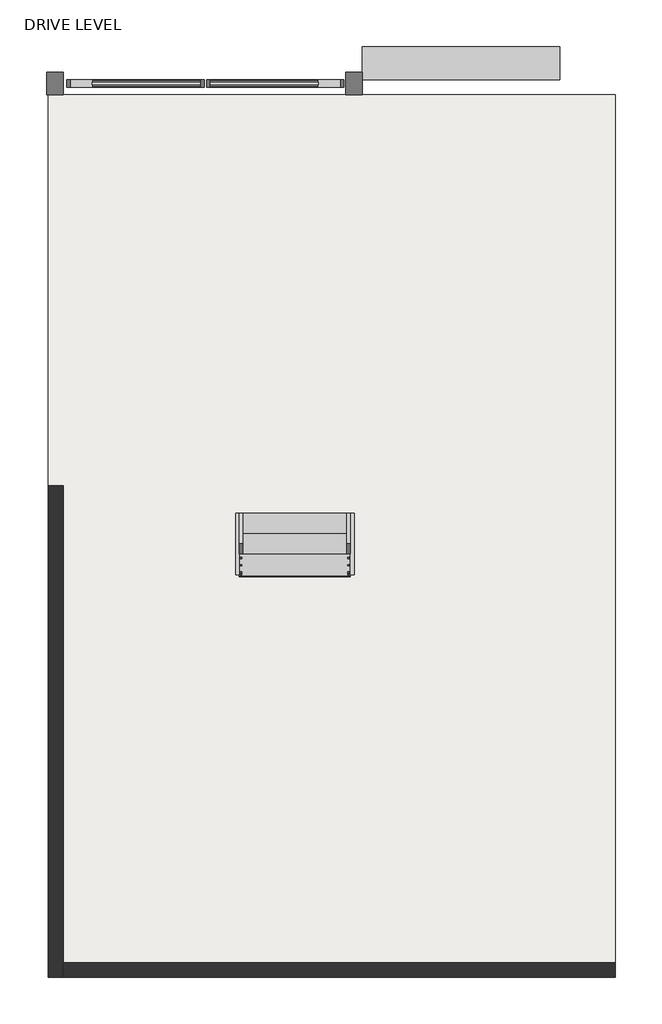
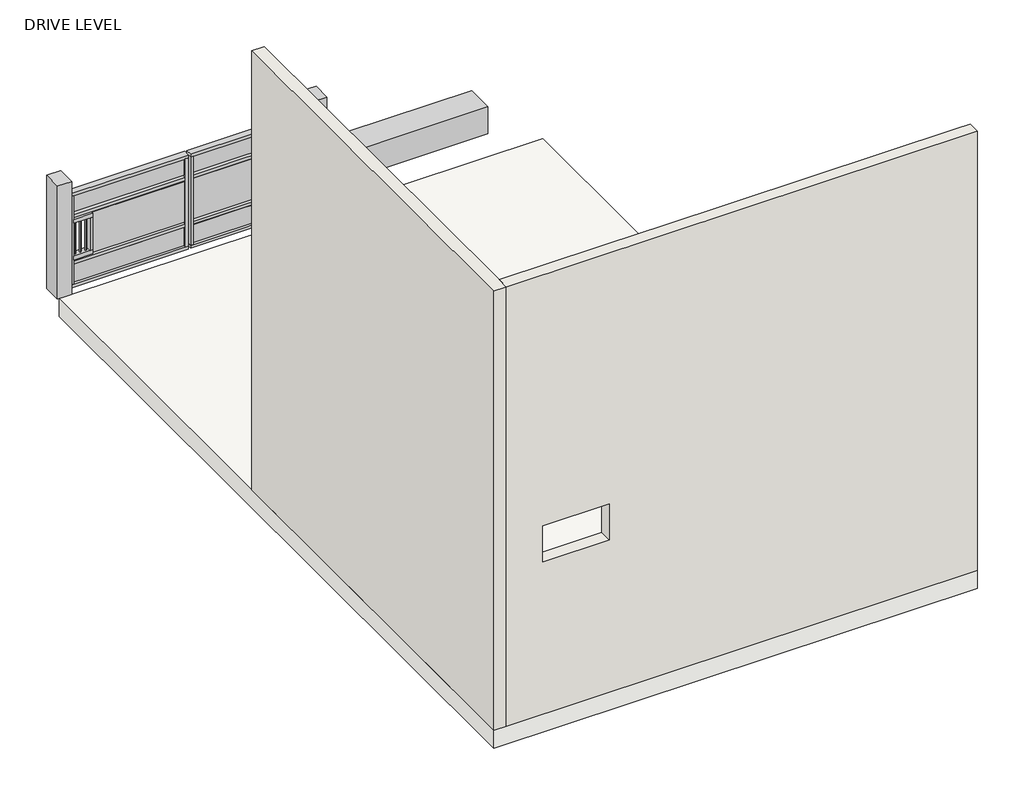
# One storey: 5 proxies, 2 members, 2 railings, 2 walls, 1 slab, 1 stair flight.
"""IFC4 building model written with IfcOpenShell, lengths in millimetres."""

from ifc_helpers import new_model, si_unit, frame, origin, place, context, project, spatial, polyline, outline, extrude, faceted_brep, transform, mapped, element, save
from components import generic_models_2_generic_models_2_050452ab, generic_models_3_generic_models_3_9be41323, generic_models_5_generic_models_3_4887dcf5, generic_models_7_generic_models_7_8565f2f4, generic_models_8_generic_models_7_bb1c0133, stair_flight_d6b1375f

model = new_model("IFC4")

# Units and contexts
model_context = context("Model", 3, world=origin())
ifc_project = project(units=[si_unit("LENGTHUNIT", "METRE", prefix="MILLI")], contexts=[model_context])

# Site, building, storey
site = spatial("IfcSite", under=ifc_project)
building = spatial("IfcBuilding", under=site)
storey = spatial("IfcBuildingStorey", under=building, Name="DRIVE LEVEL", Elevation=457.2)

# Proxies
placement = place(None, origin())
generic_models_2_generic_models_2_shape = generic_models_2_generic_models_2_050452ab(model_context)
element("IfcBuildingElementProxy", 1, Name="Generic Models 2 : Generic Models 2", ObjectType="Generic Models 2 : Generic Models 2", at=placement, inside=storey, context=model_context, shape_type="MappedRepresentation", body=[
    mapped(generic_models_2_generic_models_2_shape, transform((0.0, 0.0, 0.0), x_axis=(1.0, 0.0, 0.0), y_axis=(0.0, 1.0, 0.0), z_axis=(0.0, 0.0, 1.0))),
])
generic_models_3_generic_models_3_shape = generic_models_3_generic_models_3_9be41323(model_context)
element("IfcBuildingElementProxy", 2, Name="Generic Models 3 : Generic Models 3", ObjectType="Generic Models 3 : Generic Models 3", at=placement, inside=storey, context=model_context, shape_type="MappedRepresentation", body=[
    mapped(generic_models_3_generic_models_3_shape, transform((0.0, 0.0, 0.0), x_axis=(1.0, 0.0, 0.0), y_axis=(0.0, 1.0, 0.0), z_axis=(0.0, 0.0, 1.0))),
])
generic_models_5_generic_models_3_shape = generic_models_5_generic_models_3_4887dcf5(model_context)
element("IfcBuildingElementProxy", 3, Name="Generic Models 5 : Generic Models 3", ObjectType="Generic Models 5 : Generic Models 3", at=placement, inside=storey, context=model_context, shape_type="MappedRepresentation", body=[
    mapped(generic_models_5_generic_models_3_shape, transform((0.0, 0.0, 0.0), x_axis=(1.0, 0.0, 0.0), y_axis=(0.0, 1.0, 0.0), z_axis=(0.0, 0.0, 1.0))),
])
generic_models_7_generic_models_7_shape = generic_models_7_generic_models_7_8565f2f4(model_context)
element("IfcBuildingElementProxy", 4, Name="Generic Models 7 : Generic Models 7", ObjectType="Generic Models 7 : Generic Models 7", at=placement, inside=storey, context=model_context, shape_type="MappedRepresentation", body=[
    mapped(generic_models_7_generic_models_7_shape, transform((0.0, 0.0, 0.0), x_axis=(1.0, 0.0, 0.0), y_axis=(0.0, 1.0, 0.0), z_axis=(0.0, 0.0, 1.0))),
])
generic_models_8_generic_models_7_shape = generic_models_8_generic_models_7_bb1c0133(model_context)
element("IfcBuildingElementProxy", 5, Name="Generic Models 8 : Generic Models 7", ObjectType="Generic Models 8 : Generic Models 7", at=placement, inside=storey, context=model_context, shape_type="MappedRepresentation", body=[
    mapped(generic_models_8_generic_models_7_shape, transform((0.0, 0.0, 0.0), x_axis=(1.0, 0.0, 0.0), y_axis=(0.0, 1.0, 0.0), z_axis=(0.0, 0.0, 1.0))),
])

# Members
element("IfcMember", 6, ObjectType="Stringer - 2\" Width", at=placement, inside=storey, context=model_context, shape_type="SweptSolid", body=[
    extrude(outline(polyline([(-11301.9027976, 654.1220692), (-11301.9027976, 457.2), (-11625.5392164, 457.2), (-12140.1027976, 667.7032832), (-12140.1027976, 997.0220692), (-11301.9027976, 654.1220692)])), frame((-15545.368705, 0.0, 0.0), z_axis=(1.0, 0.0, 0.0), x_axis=(0.0, 1.0, 0.0)), (0.0, 0.0, 1.0), 50.8),
])
element("IfcMember", 7, ObjectType="Stringer - 2\" Width", at=placement, inside=storey, context=model_context, shape_type="SweptSolid", body=[
    extrude(outline(polyline([(-11301.9027976, 654.1220692), (-11301.9027976, 457.2), (-11625.5392164, 457.2), (-12140.1027976, 667.7032832), (-12140.1027976, 997.0220692), (-11301.9027976, 654.1220692)])), frame((-17120.168705, 0.0, 0.0), z_axis=(1.0, 0.0, 0.0), x_axis=(0.0, 1.0, 0.0)), (0.0, 0.0, 1.0), 50.8),
])

# Railings
element("IfcRailing", 8, ObjectType="Handrail - Rectangular", at=placement, inside=storey, context=model_context, shape_type="SweptSolid", body=[
    extrude(outline(polyline([(-11301.9027976, 1485.9), (-11301.9027976, 1431.0135357), (-12140.1027976, 1773.9135357), (-12140.1027976, 1828.8), (-11301.9027976, 1485.9)])), frame((-17069.368705, 0.0, 0.0), z_axis=(1.0, 0.0, 0.0), x_axis=(0.0, 1.0, 0.0)), (0.0, 0.0, 1.0), 50.8),
    extrude(outline(polyline([(-12124.2277976, 1767.4192175), (-12105.1777976, 1759.6260357), (-12105.1777976, 800.1), (-12124.2277976, 800.1), (-12124.2277976, 1767.4192175)])), frame((-17053.493705, 0.0, 0.0), z_axis=(1.0, 0.0, 0.0), x_axis=(0.0, 1.0, 0.0)), (0.0, 0.0, 1.0), 19.05),
    extrude(outline(polyline([(-12022.6277976, 1725.8555811), (-12003.5777976, 1718.0623993), (-12003.5777976, 800.1), (-12022.6277976, 800.1), (-12022.6277976, 1725.8555811)])), frame((-17053.493705, 0.0, 0.0), z_axis=(1.0, 0.0, 0.0), x_axis=(0.0, 1.0, 0.0)), (0.0, 0.0, 1.0), 19.05),
    extrude(outline(polyline([(-11921.0277976, 1684.2919448), (-11901.9777976, 1676.4987629), (-11901.9777976, 800.1), (-11921.0277976, 800.1), (-11921.0277976, 1684.2919448)])), frame((-17053.493705, 0.0, 0.0), z_axis=(1.0, 0.0, 0.0), x_axis=(0.0, 1.0, 0.0)), (0.0, 0.0, 1.0), 19.05),
    extrude(outline(polyline([(-11819.4277976, 1642.7283084), (-11800.3777976, 1634.9351266), (-11800.3777976, 685.8), (-11819.4277976, 685.8), (-11819.4277976, 1642.7283084)])), frame((-17053.493705, 0.0, 0.0), z_axis=(1.0, 0.0, 0.0), x_axis=(0.0, 1.0, 0.0)), (0.0, 0.0, 1.0), 19.05),
    extrude(outline(polyline([(-11717.8277976, 1601.164672), (-11698.7777976, 1593.3714902), (-11698.7777976, 685.8), (-11717.8277976, 685.8), (-11717.8277976, 1601.164672)])), frame((-17053.493705, 0.0, 0.0), z_axis=(1.0, 0.0, 0.0), x_axis=(0.0, 1.0, 0.0)), (0.0, 0.0, 1.0), 19.05),
    extrude(outline(polyline([(-11616.2277976, 1559.6010357), (-11597.1777976, 1551.8078538), (-11597.1777976, 685.8), (-11616.2277976, 685.8), (-11616.2277976, 1559.6010357)])), frame((-17053.493705, 0.0, 0.0), z_axis=(1.0, 0.0, 0.0), x_axis=(0.0, 1.0, 0.0)), (0.0, 0.0, 1.0), 19.05),
    extrude(outline(polyline([(-11514.6277976, 1518.0373993), (-11495.5777976, 1510.2442175), (-11495.5777976, 571.5), (-11514.6277976, 571.5), (-11514.6277976, 1518.0373993)])), frame((-17053.493705, 0.0, 0.0), z_axis=(1.0, 0.0, 0.0), x_axis=(0.0, 1.0, 0.0)), (0.0, 0.0, 1.0), 19.05),
    extrude(outline(polyline([(-11413.0277976, 1476.4737629), (-11393.9777976, 1468.6805811), (-11393.9777976, 571.5), (-11413.0277976, 571.5), (-11413.0277976, 1476.4737629)])), frame((-17053.493705, 0.0, 0.0), z_axis=(1.0, 0.0, 0.0), x_axis=(0.0, 1.0, 0.0)), (0.0, 0.0, 1.0), 19.05),
    extrude(outline(polyline([(-12140.1027976, 1773.9135357), (-12121.0527976, 1766.1203538), (-12121.0527976, 800.1), (-12140.1027976, 800.1), (-12140.1027976, 1773.9135357)])), frame((-17053.493705, 0.0, 0.0), z_axis=(1.0, 0.0, 0.0), x_axis=(0.0, 1.0, 0.0)), (0.0, 0.0, 1.0), 19.05),
    extrude(outline(polyline([(-11320.9527976, 1438.8067175), (-11301.9027976, 1431.0135357), (-11301.9027976, 571.5), (-11320.9527976, 571.5), (-11320.9527976, 1438.8067175)])), frame((-17053.493705, 0.0, 0.0), z_axis=(1.0, 0.0, 0.0), x_axis=(0.0, 1.0, 0.0)), (0.0, 0.0, 1.0), 19.05),
])
element("IfcRailing", 9, ObjectType="Handrail - Rectangular", at=placement, inside=storey, context=model_context, shape_type="SweptSolid", body=[
    extrude(outline(polyline([(-11301.9027976, 1485.9), (-11301.9027976, 1431.0135357), (-12140.1027976, 1773.9135357), (-12140.1027976, 1828.8), (-11301.9027976, 1485.9)])), frame((-15596.168705, 0.0, 0.0), z_axis=(1.0, 0.0, 0.0), x_axis=(0.0, 1.0, 0.0)), (0.0, 0.0, 1.0), 50.8),
    extrude(outline(polyline([(-12105.1777976, 1759.6260357), (-12105.1777976, 800.1), (-12124.2277976, 800.1), (-12124.2277976, 1767.4192175), (-12105.1777976, 1759.6260357)])), frame((-15580.293705, 0.0, 0.0), z_axis=(1.0, 0.0, 0.0), x_axis=(0.0, 1.0, 0.0)), (0.0, 0.0, 1.0), 19.05),
    extrude(outline(polyline([(-12003.5777976, 1718.0623993), (-12003.5777976, 800.1), (-12022.6277976, 800.1), (-12022.6277976, 1725.8555811), (-12003.5777976, 1718.0623993)])), frame((-15580.293705, 0.0, 0.0), z_axis=(1.0, 0.0, 0.0), x_axis=(0.0, 1.0, 0.0)), (0.0, 0.0, 1.0), 19.05),
    extrude(outline(polyline([(-11901.9777976, 1676.4987629), (-11901.9777976, 800.1), (-11921.0277976, 800.1), (-11921.0277976, 1684.2919448), (-11901.9777976, 1676.4987629)])), frame((-15580.293705, 0.0, 0.0), z_axis=(1.0, 0.0, 0.0), x_axis=(0.0, 1.0, 0.0)), (0.0, 0.0, 1.0), 19.05),
    extrude(outline(polyline([(-11800.3777976, 1634.9351266), (-11800.3777976, 685.8), (-11819.4277976, 685.8), (-11819.4277976, 1642.7283084), (-11800.3777976, 1634.9351266)])), frame((-15580.293705, 0.0, 0.0), z_axis=(1.0, 0.0, 0.0), x_axis=(0.0, 1.0, 0.0)), (0.0, 0.0, 1.0), 19.05),
    extrude(outline(polyline([(-11698.7777976, 1593.3714902), (-11698.7777976, 685.8), (-11717.8277976, 685.8), (-11717.8277976, 1601.164672), (-11698.7777976, 1593.3714902)])), frame((-15580.293705, 0.0, 0.0), z_axis=(1.0, 0.0, 0.0), x_axis=(0.0, 1.0, 0.0)), (0.0, 0.0, 1.0), 19.05),
    extrude(outline(polyline([(-11597.1777976, 1551.8078538), (-11597.1777976, 685.8), (-11616.2277976, 685.8), (-11616.2277976, 1559.6010357), (-11597.1777976, 1551.8078538)])), frame((-15580.293705, 0.0, 0.0), z_axis=(1.0, 0.0, 0.0), x_axis=(0.0, 1.0, 0.0)), (0.0, 0.0, 1.0), 19.05),
    extrude(outline(polyline([(-11495.5777976, 1510.2442175), (-11495.5777976, 571.5), (-11514.6277976, 571.5), (-11514.6277976, 1518.0373993), (-11495.5777976, 1510.2442175)])), frame((-15580.293705, 0.0, 0.0), z_axis=(1.0, 0.0, 0.0), x_axis=(0.0, 1.0, 0.0)), (0.0, 0.0, 1.0), 19.05),
    extrude(outline(polyline([(-11393.9777976, 1468.6805811), (-11393.9777976, 571.5), (-11413.0277976, 571.5), (-11413.0277976, 1476.4737629), (-11393.9777976, 1468.6805811)])), frame((-15580.293705, 0.0, 0.0), z_axis=(1.0, 0.0, 0.0), x_axis=(0.0, 1.0, 0.0)), (0.0, 0.0, 1.0), 19.05),
    extrude(outline(polyline([(-12121.0527976, 1766.1203538), (-12121.0527976, 800.1), (-12140.1027976, 800.1), (-12140.1027976, 1773.9135357), (-12121.0527976, 1766.1203538)])), frame((-15580.293705, 0.0, 0.0), z_axis=(1.0, 0.0, 0.0), x_axis=(0.0, 1.0, 0.0)), (0.0, 0.0, 1.0), 19.05),
    extrude(outline(polyline([(-11301.9027976, 1431.0135357), (-11301.9027976, 571.5), (-11320.9527976, 571.5), (-11320.9527976, 1438.8067175), (-11301.9027976, 1431.0135357)])), frame((-15580.293705, 0.0, 0.0), z_axis=(1.0, 0.0, 0.0), x_axis=(0.0, 1.0, 0.0)), (0.0, 0.0, 1.0), 19.05),
])

# Slab
element("IfcSlab", 10, ObjectType="Generic - 12\"", at=placement, inside=storey, context=model_context, shape_type="SweptSolid", body=[
    extrude(outline(polyline([(-11913.168705, -5561.5027976), (-11913.168705, -17664.6027976), (-19685.568705, -17664.6027976), (-19685.568705, -5561.5027976), (-11913.168705, -5561.5027976)])), frame((0.0, 0.0, 152.4), z_axis=(0.0, 0.0, 1.0), x_axis=(1.0, 0.0, 0.0)), (0.0, 0.0, 1.0), 304.8),
])

# Stair flight
stair_flight_shape = stair_flight_d6b1375f(model_context)
element("IfcStairFlight", 11, ObjectType="2\" Tread 1\" Nosing 1/4\" Riser", at=placement, inside=storey, context=model_context, shape_type="MappedRepresentation", body=[
    mapped(stair_flight_shape, transform((0.0, 0.0, 0.0), x_axis=(1.0, 0.0, 0.0), y_axis=(0.0, 1.0, 0.0), z_axis=(0.0, 0.0, 1.0))),
])

# Walls
element("IfcWall", 12, ObjectType="Generic - 8\"", at=placement, inside=storey, context=model_context, shape_type="Brep", body=[
    faceted_brep([(-19685.568705, -10920.9027976, 457.2), (-19685.568705, -17664.6027976, 457.2), (-19685.568705, -17664.6027976, 7924.8), (-19685.568705, -10920.9027976, 7924.8), (-19685.568705, -10920.9027976, 2286.0), (-19482.368705, -10920.9027976, 457.2), (-19482.368705, -10920.9027976, 2286.0), (-19482.368705, -10920.9027976, 7924.8), (-19482.368705, -17461.4027976, 7924.8), (-19482.368705, -17664.6027976, 7924.8), (-19482.368705, -17664.6027976, 457.2), (-19482.368705, -17461.4027976, 457.2)], [[[0, 1, 2, 3, 4]], [[5, 6, 7, 8, 9, 10, 11]], [[1, 0, 5, 11, 10]], [[3, 2, 9, 8, 7]], [[0, 4, 3, 7, 6, 5]], [[2, 1, 10, 9]]]),
])
element("IfcWall", 13, ObjectType="Generic - 8\"", at=placement, inside=storey, context=model_context, shape_type="Brep", body=[
    faceted_brep([(-19482.368705, -17664.6027976, 457.2), (-11913.168705, -17664.6027976, 457.2), (-11913.168705, -17664.6027976, 7924.8), (-19482.368705, -17664.6027976, 7924.8), (-17831.368705, -17664.6027976, 3657.6), (-17831.368705, -17664.6027976, 3048.0), (-18898.168705, -17664.6027976, 3048.0), (-18898.168705, -17664.6027976, 3657.6), (-19482.368705, -17461.4027976, 457.2), (-19482.368705, -17461.4027976, 7924.8), (-17120.168705, -17461.4027976, 7924.8), (-16916.968705, -17461.4027976, 7924.8), (-12116.368705, -17461.4027976, 7924.8), (-11913.168705, -17461.4027976, 7924.8), (-11913.168705, -17461.4027976, 914.4), (-11913.168705, -17461.4027976, 457.2), (-17831.368705, -17461.4027976, 3657.6), (-18898.168705, -17461.4027976, 3657.6), (-18898.168705, -17461.4027976, 3048.0), (-17831.368705, -17461.4027976, 3048.0)], [[[0, 1, 2, 3], [4, 5, 6, 7]], [[8, 9, 10, 11, 12, 13, 14, 15], [16, 17, 18, 19]], [[1, 0, 8, 15]], [[3, 2, 13, 12, 11, 10, 9]], [[0, 3, 9, 8]], [[2, 1, 15, 14, 13]], [[5, 4, 16, 19]], [[6, 5, 19, 18]], [[7, 6, 18, 17]], [[4, 7, 17, 16]]]),
])

save(model, "model.ifc")

# Revit data of these elements
# Type "Handrail - Rectangular"
#   Assembly Code = "C2010400"
#   built-in parameter 1008612 = 0.0416667 (stored number, unit not read)
#   built-in parameter 1008611 = 0.0416667 (stored number, unit not read)
#   built-in parameter 1008609 = 0.333333 (stored number, unit not read)
#   built-in parameter 1008604 = 0.166667 (stored number, unit not read)
#   built-in parameter 1008603 = 0.166667 (stored number, unit not read)
#   Railing Height = 3' - 0"
#   built-in parameter 1008630 = 2
#   built-in parameter 1008610 = 2
#   built-in parameter 1008618 = Baluster - Square : 3/4"
# Type "Generic - 12\""
#   Assembly Code = "B1010"
#   Function = 0
#   Layers, outside or top first: 1' - 0" no material (function 1)
# Type "Generic - 8\""
#   Assembly Code = "B2010"
#   Layers, outside or top first: 0' - 8" no material (function 1)
# Element 1 (IfcBuildingElementProxy, "Generic Models 2 : Generic Models 2")
#   Phase Created = New Construction
#   Materials on its faces: "Gypsum Wall Board"
# Element 2 (IfcBuildingElementProxy, "Generic Models 3 : Generic Models 3")
#   Phase Created = New Construction
# Element 3 (IfcBuildingElementProxy, "Generic Models 5 : Generic Models 3")
#   Phase Created = New Construction
# Element 4 (IfcBuildingElementProxy, "Generic Models 7 : Generic Models 7")
#   Phase Created = New Construction
#   Materials on its faces: "Damp-proofing", "Gypsum Wall Board", "Wood Planks"
# Element 5 (IfcBuildingElementProxy, "Generic Models 8 : Generic Models 7")
#   Phase Created = New Construction
#   Materials on its faces: "Damp-proofing", "Gypsum Wall Board", "Wood Planks"
# Elements 6, 7 (IfcMember, "Stringer - 2\" Width")
#   Phase Created = New Construction
# Elements 8, 9 (IfcRailing, "Handrail - Rectangular")
#   Phase Created = New Construction
# Element 10 (IfcSlab, "Generic - 12\"")
#   Height Offset From Level = 0' - 0"
#   Phase Created = New Construction
#   Materials on its faces: "Default Floor"
# Element 11 (IfcStairFlight, "2\" Tread 1\" Nosing 1/4\" Riser")
#   Phase Created = New Construction
# Elements 12, 13 (IfcWall, "Generic - 8\"")
#   Top Offset = 0' - 0"
#   Base Offset = 0' - 0"
#   wall height = 24' - 6"
#   Phase Created = New Construction
#   Base Constraint = DRIVE LEVEL
#   Top Constraint = ROOF LEVEL
#   Materials on its faces: "Default Wall"
# Materials
#   "Gypsum Wall Board": class "Generic", colour RGB 228 228 228, transparency 0, Description = "Gypsum Wall Board", Cost = 0
#   "Damp-proofing": class "Generic", colour RGB 17 17 17, transparency 0, Description = "Damp-proofing", Cost = 0
#   "Wood Planks": class "Wood", colour RGB 129 72 39, transparency 0, Description = "Physical material.", Cost = 0
#   "Default Floor": colour RGB 128 128 128, transparency 0, Cost = 0
#   "Default Wall": colour RGB 128 128 128, transparency 0, Cost = 0
